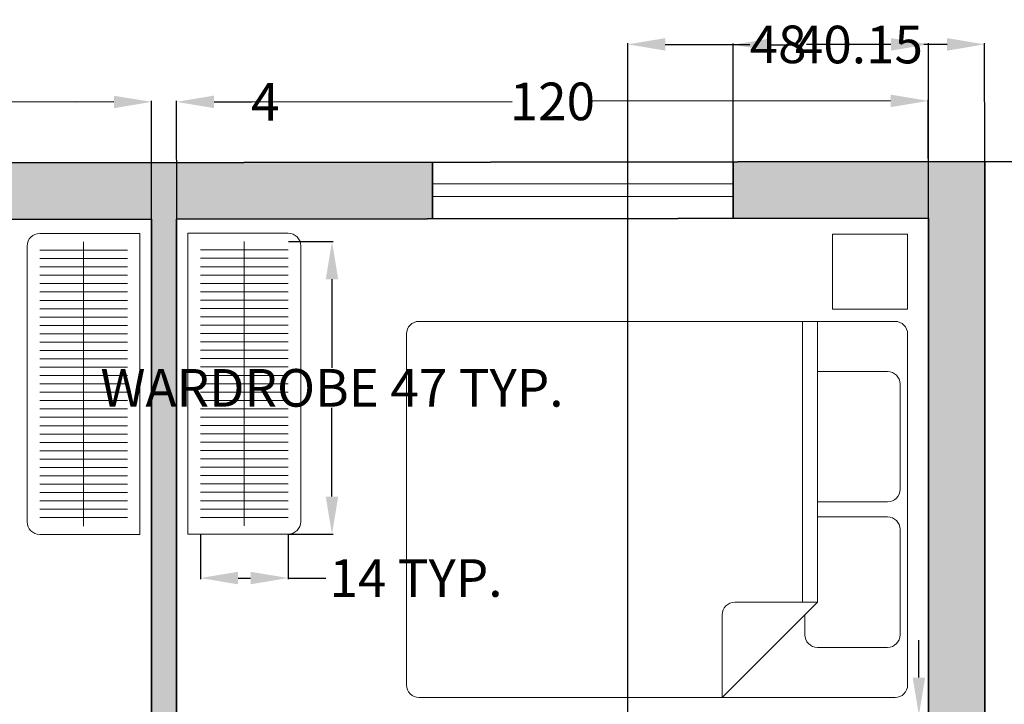
# Model space of a CAD drawing. Units: inches. Extents: x 98 to 487, y -240 to 141.
# Tile 4 of 5: x 251 to 408, y 32 to 141. Entities that reach past the tile are written whole.
import ezdxf

# ---------------------------------------------------------------- set-up
doc = ezdxf.new("R2010")
doc.units = ezdxf.units.IN
doc.header["$MEASUREMENT"] = 0
for name, color, linetype, lineweight in [('A-ANNO-DIMS', 2, 'Continuous', 18), ('A-FURN', 8, 'Continuous', 18), ('A-GLAZ', 4, 'Continuous', 18), ('A-WALL', 7, 'Continuous', 35)]:
    doc.layers.add(name, color=color, linetype=linetype, lineweight=lineweight)
doc.layers.add('A-WALL-PATT', color=251, linetype='Continuous', lineweight=13, true_color=0x636466)
doc.styles.get("Standard").update_dxf_attribs({"font": 'arial.ttf'})
doc.dimstyles.get("Standard").update_dxf_attribs({"dimtxt": 6, "dimasz": 6, "dimexe": 0.18, "dimexo": 0.0625, "dimgap": 0.09, "dimtad": 0, "dimtih": 1, "dimtoh": 1, "dimdec": 0, "dimzin": 0, "dimdsep": 46, "dimlunit": 4, "dimtxsty": 'Standard', "dimcen": 0.09, "dimadec": 0, "dimazin": 0, "dimtfac": 1, "dimtdec": 0, "dimtofl": 0, "dimtmove": 0, "dimatfit": 3, "dimfxl": 1, "dimtolj": 1, "dimtzin": 0, "dimarcsym": 0})

# ---------------------------------------------------------------- blocks, each defined once
blk = doc.blocks.new('Bed - Queen')
for p, q in [((2, 0), (57.99999, 0)), ((9.99999, -1.2), (26.79998, -1.2)), ((33.19999, -1.2), (49.99999, -1.2)), ((0, -78.00003), (0, -2)), ((59.99999, -2), (59.99999, -78.00003)), ((7.99999, -14.4), (7.99999, -3.2)), ((28.79998, -3.2), (28.79998, -14.4)), ((31.19999, -14.4), (31.19999, -3.2)), ((51.99999, -3.2), (51.99999, -14.4)), ((0, -14.4), (44.8, -14.4)), ((59.99999, -29.6), (44.8, -14.4)), ((44.8, -14.4), (44.8, -27.6)), ((44.8, -16.8), (0, -16.8)), ((49.99999, -16.4), (46.79936, -16.4)), ((46.8, -29.6), (59.99999, -29.6)), ((57.99999, -80.00003), (2, -80.00003))]:
    blk.add_line(p, q)
for centre, start, end in [((2, -2), 90, 180), ((57.99999, -2), 0, 90), ((9.99999, -3.2), 90, 180), ((26.79998, -3.2), 0, 90), ((33.19999, -3.2), 90, 180), ((49.99999, -3.2), 0, 90), ((49.99999, -14.4), 270, 0), ((46.8, -27.6), 180, 270), ((2, -78.00003), 180, 270), ((57.99999, -78.00003), 270, 0)]:
    blk.add_arc(centre, 2, start, end)
blk = doc.blocks.new('GLAZ-48IN')
for p, q in [((48, 2), (0, 2)), ((48, 0), (0, 0))]:
    blk.add_line(p, q)
blk = doc.blocks.new('NIGHTSTAND-12IN-SQUARE')
blk.add_lwpolyline([(12, 12), (0, 12), (0, 0), (12, 0)], close=True)
blk = doc.blocks.new('WARDROBE-HANGING-RAIL')
for p, q in [((7, 46.67), (7, 1.33)), ((14, 45.33), (0, 45.33)), ((14, 44), (0, 44)), ((14, 42.67), (0, 42.67)), ((14, 41.33), (0, 41.33)), ((14, 40), (0, 40)), ((14, 38.67), (0, 38.67)), ((14, 37.33), (0, 37.33)), ((14, 36), (0, 36)), ((14, 34.67), (0, 34.67)), ((14, 33.33), (0, 33.33)), ((14, 32), (0, 32)), ((14, 30.67), (0, 30.67)), ((14, 29.33), (0, 29.33)), ((14, 28), (0, 28)), ((14, 26.67), (0, 26.67)), ((14, 25.33), (0, 25.33)), ((14, 24), (0, 24)), ((14, 22.67), (0, 22.67)), ((14, 21.33), (0, 21.33)), ((14, 20), (0, 20)), ((14, 18.67), (0, 18.67)), ((14, 17.33), (0, 17.33)), ((14, 16), (0, 16)), ((14, 14.67), (0, 14.67)), ((14, 13.33), (0, 13.33)), ((14, 12), (0, 12)), ((14, 10.67), (0, 10.67)), ((14, 9.33), (0, 9.33)), ((14, 8), (0, 8)), ((14, 6.67), (0, 6.67)), ((14, 5.33), (0, 5.33)), ((14, 4), (0, 4)), ((14, 2.67), (0, 2.67)), ((14, 0), (0, 0))]:
    blk.add_line(p, q)
blk = doc.blocks.new('*D22')
at = {"layer": 'A-ANNO-DIMS', "color": 0, "lineweight": -2, "transparency": 16777216}
for p, q in [((293.63, 105.87), (300.74, 105.87)), ((300.56, 99.87), (300.56, 85.73)), ((300.56, 65.2), (300.56, 79.34)), ((293.63, 59.2), (300.74, 59.2))]:
    blk.add_line(p, q, dxfattribs=at)
at = {"layer": 'A-ANNO-DIMS', "color": 0, "transparency": 16777216}
for points in [[(299.56, 99.87), (301.56, 99.87), (300.56, 105.87)], [(299.56, 65.2), (301.56, 65.2), (300.56, 59.2)]]:
    blk.add_solid(points, dxfattribs=at)
at = {"layer": 'Defpoints', "color": 0, "transparency": 16777216}
for p in [(293.56, 105.87), (300.56, 105.87), (293.56, 59.2)]:
    blk.add_point(p, dxfattribs=at)
at = {"layer": 'A-ANNO-DIMS', "color": 0, "transparency": 16777216, "insert": (300.56, 82.54), "char_height": 6, "attachment_point": 5}
blk.add_mtext('\\A1;WARDROBE 47 TYP.', dxfattribs=at)
blk = doc.blocks.new('*D23')
at = {"layer": 'A-ANNO-DIMS', "color": 0, "lineweight": -2, "transparency": 16777216}
for p, q in [((279.56, 59.14), (279.56, 52.02)), ((293.56, 59.14), (293.56, 52.02)), ((285.56, 52.2), (287.56, 52.2)), ((293.56, 52.2), (299.56, 52.2))]:
    blk.add_line(p, q, dxfattribs=at)
at = {"layer": 'A-ANNO-DIMS', "color": 0, "transparency": 16777216}
for points in [[(285.56, 53.2), (285.56, 51.2), (279.56, 52.2)], [(287.56, 53.2), (287.56, 51.2), (293.56, 52.2)]]:
    blk.add_solid(points, dxfattribs=at)
at = {"layer": 'Defpoints', "color": 0, "transparency": 16777216}
for p in [(279.56, 59.2), (293.56, 59.2), (293.56, 52.2)]:
    blk.add_point(p, dxfattribs=at)
at = {"layer": 'A-ANNO-DIMS', "color": 0, "transparency": 16777216, "insert": (313.97, 52.2), "char_height": 6, "attachment_point": 5}
blk.add_mtext('\\A1;14 TYP.', dxfattribs=at)
blk = doc.blocks.new('*D27')
at = {"layer": 'A-ANNO-DIMS', "color": 0, "lineweight": -2, "transparency": 16777216}
for p, q in [((394.25, 36.31), (394.25, 42.31)), ((392.51, 30.31), (394.43, 30.31)), ((392.51, 18.31), (394.43, 18.31)), ((394.25, 12.31), (394.25, 6.31))]:
    blk.add_line(p, q, dxfattribs=at)
at = {"layer": 'A-ANNO-DIMS', "color": 0, "transparency": 16777216}
for points in [[(393.25, 36.31), (395.25, 36.31), (394.25, 30.31)], [(393.25, 12.31), (395.25, 12.31), (394.25, 18.31)]]:
    blk.add_solid(points, dxfattribs=at)
at = {"layer": 'Defpoints', "color": 0, "transparency": 16777216}
for p in [(392.45, 30.31), (394.25, 30.31), (392.45, 18.31)]:
    blk.add_point(p, dxfattribs=at)
at = {"layer": 'A-ANNO-DIMS', "color": 0, "transparency": 16777216, "insert": (394.25, 24.31), "char_height": 6, "attachment_point": 5}
blk.add_mtext('\\A1;12 TYP.', dxfattribs=at)
blk = doc.blocks.new('*D47')
at = {"layer": 'A-ANNO-DIMS', "color": 0, "lineweight": -2, "transparency": 16777216}
for p, q in [((404.83, 118.64), (423.65, 118.64)), ((423.47, 112.64), (423.47, -46.22)), ((423.47, -211.38), (423.47, -52.53)), ((404.83, -217.38), (423.65, -217.38))]:
    blk.add_line(p, q, dxfattribs=at)
at = {"layer": 'A-ANNO-DIMS', "color": 0, "transparency": 16777216}
for points in [[(422.47, 112.64), (424.47, 112.64), (423.47, 118.64)], [(422.47, -211.38), (424.47, -211.38), (423.47, -217.38)]]:
    blk.add_solid(points, dxfattribs=at)
at = {"layer": 'Defpoints', "color": 0, "transparency": 16777216}
for p in [(404.77, 118.64), (404.77, -217.38), (423.47, -217.38)]:
    blk.add_point(p, dxfattribs=at)
at = {"layer": 'A-ANNO-DIMS', "color": 0, "transparency": 16777216, "insert": (423.47, -49.37), "char_height": 6, "attachment_point": 5}
blk.add_mtext('\\A1;336', dxfattribs=at)
blk = doc.blocks.new('*D49')
at = {"layer": 'A-ANNO-DIMS', "color": 0, "lineweight": -2, "transparency": 16777216}
for p, q in [((364.62, 118.64), (364.59, 137.46)), ((370.59, 137.29), (374.31, 137.29)), ((398.74, 137.33), (395.02, 137.32)), ((404.77, 118.7), (404.74, 137.52))]:
    blk.add_line(p, q, dxfattribs=at)
at = {"layer": 'A-ANNO-DIMS', "color": 0, "transparency": 16777216}
for points in [[(398.74, 138.33), (398.74, 136.33), (404.74, 137.34)], [(370.59, 138.29), (370.59, 136.29), (364.59, 137.28)]]:
    blk.add_solid(points, dxfattribs=at)
at = {"layer": 'Defpoints', "color": 0, "transparency": 16777216}
for p in [(404.74, 137.34), (364.62, 118.58), (404.77, 118.64)]:
    blk.add_point(p, dxfattribs=at)
at = {"layer": 'A-ANNO-DIMS', "color": 0, "transparency": 16777216, "insert": (384.67, 137.31), "char_height": 6, "attachment_point": 5}
blk.add_mtext('\\A1;40.15', dxfattribs=at)
blk = doc.blocks.new('*D50')
at = {"layer": 'A-ANNO-DIMS', "color": 0, "lineweight": -2, "transparency": 16777216}
for p, q in [((137.77, 109.34), (137.74, 128.16)), ((143.74, 127.99), (198.32, 128.06)), ((265.74, 128.15), (211.16, 128.08)), ((271.77, 109.52), (271.74, 128.34))]:
    blk.add_line(p, q, dxfattribs=at)
at = {"layer": 'A-ANNO-DIMS', "color": 0, "transparency": 16777216}
for points in [[(143.74, 128.99), (143.74, 126.99), (137.74, 127.98)], [(265.74, 129.15), (265.74, 127.15), (271.74, 128.16)]]:
    blk.add_solid(points, dxfattribs=at)
at = {"layer": 'Defpoints', "color": 0, "transparency": 16777216}
for p in [(271.74, 128.16), (137.77, 109.28), (271.77, 109.46)]:
    blk.add_point(p, dxfattribs=at)
at = {"layer": 'A-ANNO-DIMS', "color": 0, "transparency": 16777216, "insert": (204.74, 128.07), "char_height": 6, "attachment_point": 5}
blk.add_mtext('\\A1;134', dxfattribs=at)
blk = doc.blocks.new('*D51')
at = {"layer": 'A-ANNO-DIMS', "color": 0, "lineweight": -2, "transparency": 16777216}
for p, q in [((265.74, 128.15), (259.74, 128.14)), ((271.77, 109.52), (271.74, 128.34)), ((275.77, 109.53), (275.74, 128.34)), ((281.74, 128.17), (287.74, 128.18))]:
    blk.add_line(p, q, dxfattribs=at)
at = {"layer": 'A-ANNO-DIMS', "color": 0, "transparency": 16777216}
for points in [[(265.74, 129.15), (265.74, 127.15), (271.74, 128.16)], [(281.74, 129.17), (281.74, 127.17), (275.74, 128.16)]]:
    blk.add_solid(points, dxfattribs=at)
at = {"layer": 'Defpoints', "color": 0, "transparency": 16777216}
for p in [(275.74, 128.16), (271.77, 109.46), (275.77, 109.46)]:
    blk.add_point(p, dxfattribs=at)
at = {"layer": 'A-ANNO-DIMS', "color": 0, "transparency": 16777216, "insert": (289.91, 128.18), "char_height": 6, "attachment_point": 5}
blk.add_mtext('\\A1;4', dxfattribs=at)
blk = doc.blocks.new('*D52')
at = {"layer": 'A-ANNO-DIMS', "color": 0, "lineweight": -2, "transparency": 16777216}
for p, q in [((275.77, 109.53), (275.74, 128.34)), ((281.74, 128.17), (329.32, 128.23)), ((389.74, 128.32), (342.17, 128.25)), ((395.77, 109.69), (395.74, 128.5))]:
    blk.add_line(p, q, dxfattribs=at)
at = {"layer": 'A-ANNO-DIMS', "color": 0, "transparency": 16777216}
for points in [[(281.74, 129.17), (281.74, 127.17), (275.74, 128.16)], [(389.74, 129.32), (389.74, 127.32), (395.74, 128.32)]]:
    blk.add_solid(points, dxfattribs=at)
at = {"layer": 'Defpoints', "color": 0, "transparency": 16777216}
for p in [(395.74, 128.32), (275.77, 109.46), (395.77, 109.62)]:
    blk.add_point(p, dxfattribs=at)
at = {"layer": 'A-ANNO-DIMS', "color": 0, "transparency": 16777216, "insert": (335.74, 128.24), "char_height": 6, "attachment_point": 5}
blk.add_mtext('\\A1;120', dxfattribs=at)
blk = doc.blocks.new('*D67')
at = {"layer": 'A-ANNO-DIMS', "color": 0, "lineweight": -2, "transparency": 16777216}
for p, q in [((347.77, 9.62), (347.77, 137.52)), ((353.77, 137.34), (367.25, 137.34)), ((389.77, 137.34), (376.28, 137.34)), ((395.77, 9.69), (395.77, 137.52))]:
    blk.add_line(p, q, dxfattribs=at)
at = {"layer": 'A-ANNO-DIMS', "color": 0, "transparency": 16777216}
for points in [[(353.77, 138.34), (353.77, 136.34), (347.77, 137.34)], [(389.77, 138.34), (389.77, 136.34), (395.77, 137.34)]]:
    blk.add_solid(points, dxfattribs=at)
at = {"layer": 'Defpoints', "color": 0, "transparency": 16777216}
for p in [(395.77, 137.34), (347.77, 9.56), (395.77, 9.62)]:
    blk.add_point(p, dxfattribs=at)
at = {"layer": 'A-ANNO-DIMS', "color": 0, "transparency": 16777216, "insert": (371.77, 137.34), "char_height": 6, "attachment_point": 5}
blk.add_mtext('\\A1;48', dxfattribs=at)

msp = doc.modelspace()

# ---------------------------------------------------------------- hatches: boundary and pattern name
at = {"layer": 'A-WALL-PATT'}
h = msp.add_hatch(color=256, dxfattribs=at)
h.dxf.hatch_style = 1
h.paths.add_polyline_path([(316.6174, 118.5177), (214.5584, 118.3815), (214.5584, 109.3815), (271.7663, 109.4578), (271.7663, 13.4577), (265.7717, 13.4497), (265.7717, 9.4497), (271.7663, 9.4577), (281.7716, 9.4711), (281.7663, 13.4711), (275.7663, 13.4631), (275.7663, 109.4632), (316.6174, 109.5177)])
h = msp.add_hatch(color=256, dxfattribs=at)
h.dxf.hatch_style = 1
h.paths.add_polyline_path([(404.7663, 118.6353), (364.6174, 118.5817), (364.6174, 109.5817), (395.7663, 109.6233), (395.7663, 13.6232), (311.7663, 13.5111), (311.7716, 9.5111), (343.7663, 9.5538), (343.7663, -2.4462), (347.7663, -2.4409), (347.7663, 9.5591), (395.7663, 9.6232), (395.7663, -2.698), (404.7663, -2.698)])

# ---------------------------------------------------------------- linework, layer by layer
at = {"layer": 'A-FURN'}
for p, q in [((277.5627, 59.2036), (277.5627, 107.2036)), ((277.5627, 107.2036), (293.5627, 107.2036)), ((295.5627, 105.2036), (295.5627, 61.2036)), ((293.5627, 59.2036), (277.5627, 59.2036))]:
    msp.add_line(p, q, dxfattribs=at)
msp.add_lwpolyline([(269.9075, 107.1706), (269.9075, 59.1706), (253.9075, 59.1706, -0.41421356), (251.9075, 61.1706), (251.9075, 105.1706, -0.41421356), (253.9075, 107.1706)], format="xyb", close=True, dxfattribs=at)
for centre, start, end in [((293.5627, 105.2036), 0, 90), ((293.5627, 61.2036), 270, 0)]:
    msp.add_arc(centre, 2, start, end, dxfattribs=at)
at = {"layer": 'A-WALL'}
for p, q in [((316.6174, 109.5817), (316.6174, 118.5817)), ((364.6174, 118.5817), (364.6174, 109.5817)), ((137.7655, 109.2791), (271.7663, 109.4578)), ((271.7663, 109.4578), (271.7663, 13.4577)), ((275.7663, 109.4632), (395.7663, 109.6233)), ((275.7663, 109.4632), (275.7663, 13.4631)), ((395.7663, 109.6233), (395.7663, 13.6232))]:
    msp.add_line(p, q, dxfattribs=at)
msp.add_lwpolyline([(143.7775, -181.7129), (128.7655, -181.7329), (128.7655, 118.2671), (404.7663, 118.6353), (404.7663, -181.3647)], dxfattribs=at)

# ---------------------------------------------------------------- block references
at = {"layer": 'A-FURN'}
for name, p in [('NIGHTSTAND-12IN-SQUARE', (380.446, 95.0694)), ('WARDROBE-HANGING-RAIL', (253.908, 59.171)), ('WARDROBE-HANGING-RAIL', (279.5632, 59.204))]:
    msp.add_blockref(name, p, dxfattribs=at)
at = {"layer": 'A-FURN', "rotation": 270}
msp.add_blockref('Bed - Queen', (392.4456, 93.1451), dxfattribs=at)
at = {"layer": 'A-GLAZ'}
msp.add_blockref('GLAZ-48IN', (316.617, 113.0822), dxfattribs=at)

# ---------------------------------------------------------------- dimensions: what is measured, and where the dimension line sits
at = {"layer": 'A-ANNO-DIMS'}
dim = msp.add_linear_dim(base=(395.7663, 137.3353), p1=(347.7663, 9.5591), p2=(395.7663, 9.6232), dimstyle='Standard', override={"dimdec": 0, "dimlfac": 1, "dimrnd": 0, "dimzin": 0, "dimdsep": 46, "dimlunit": 2}, dxfattribs=at)
dim.commit()
dim.dimension.update_dxf_attribs({"geometry": '*D67', "text_midpoint": (371.7663, 137.3353)})
for base, p1, p2, angle, override, picture, middle in [((404.7413, 137.3353), (364.6174, 118.5817), (404.7663, 118.6353), 0.076451, {"dimdec": 2, "dimlfac": 1, "dimrnd": 0, "dimzin": 0, "dimdsep": 46, "dimlunit": 2}, '*D49', (384.6669, 137.3085)), ((275.7414, 128.1631), (271.7663, 109.4578), (275.7663, 109.4632), 0.07644, {"dimdec": 0, "dimlfac": 1, "dimrnd": 0, "dimzin": 0, "dimdsep": 46, "dimlunit": 2}, '*D51', (289.9064, 128.1792)), ((395.7414, 128.3232), (275.7663, 109.4632), (395.7663, 109.6233), 0.07644, {"dimdec": 0, "dimlfac": 1, "dimrnd": 0, "dimzin": 0, "dimdsep": 46, "dimlunit": 2}, '*D52', (335.7414, 128.2432)), ((271.7414, 128.1578), (137.7655, 109.2791), (271.7663, 109.4578), 0.07644, {"dimdec": 0, "dimlfac": 1, "dimrnd": 0, "dimzin": 0, "dimdsep": 46, "dimlunit": 2}, '*D50', (204.7409, 128.0684)), ((423.4663, -217.3767), (404.7663, 118.6353), (404.7663, -217.3767), 90, {"dimdec": 0, "dimlfac": 1, "dimrnd": 0, "dimzin": 0, "dimdsep": 46, "dimlunit": 2}, '*D47', (423.4663, -49.3707))]:
    dim = msp.add_linear_dim(base=base, p1=p1, p2=p2, angle=angle, dimstyle='Standard', override=override, dxfattribs=at)
    dim.commit()
    dim.dimension.update_dxf_attribs({"geometry": picture, "text_midpoint": middle})
for base, p1, p2, text, picture, middle in [((300.5627, 105.8702), (293.5627, 59.2036), (293.5627, 105.8702), 'WARDROBE <> TYP.', '*D22', (300.5627, 82.5369)), ((394.2456, 30.3145), (392.4456, 18.3145), (392.4456, 30.3145), '<> TYP.', '*D27', (394.2456, 24.3145))]:
    dim = msp.add_linear_dim(base=base, p1=p1, p2=p2, angle=90, text=text, dimstyle='Standard', override={"dimdec": 0, "dimlfac": 1, "dimrnd": 0, "dimzin": 0, "dimdsep": 46, "dimlunit": 2}, dxfattribs=at)
    dim.commit()
    dim.dimension.update_dxf_attribs({"geometry": picture, "text_midpoint": middle})
dim = msp.add_linear_dim(base=(293.5627, 52.2036), p1=(279.5627, 59.2036), p2=(293.5627, 59.2036), text='<> TYP.', dimstyle='Standard', override={"dimdec": 0, "dimlfac": 1, "dimrnd": 0, "dimzin": 0, "dimdsep": 46, "dimlunit": 2}, dxfattribs=at)
dim.commit()
dim.dimension.update_dxf_attribs({"geometry": '*D23', "text_midpoint": (313.9733, 52.2036)})

doc.saveas('drawing.dxf')
